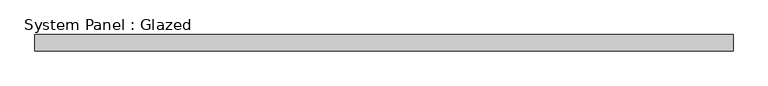
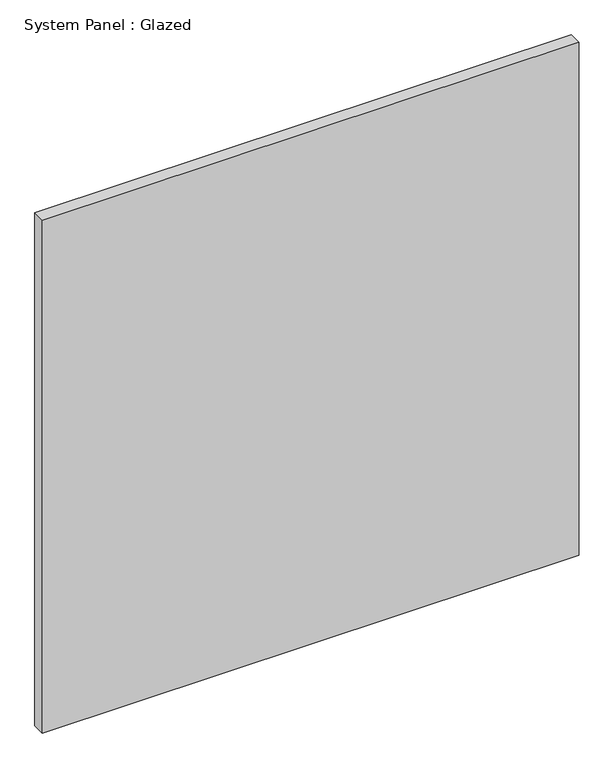
"""IFC4 building model written with IfcOpenShell, lengths in millimetres: plate geometry, System Panel : Glazed."""

from ifc_helpers import new_model, si_unit, origin, origin_with_axes, place, context, project, spatial, polyline, outline, extrude, source, transform, mapped, element, save


def system_panel_glazed_bea6ef26(model_context):
    return source(origin(), model_context, "Body", "SweptSolid", [
        extrude(outline(polyline([(528.0, 24.5), (-528.0, 24.5), (-528.0, 49.5), (528.0, 49.5), (528.0, 24.5)])), origin_with_axes(), (0.0, 0.0, 1.0), 1066.8),
    ])


if __name__ == "__main__":
    model = new_model("IFC4")
    model_context = context("Model", 3, world=origin())
    ifc_project = project(units=[si_unit("LENGTHUNIT", "METRE", prefix="MILLI")], contexts=[model_context])
    site = spatial("IfcSite", under=ifc_project)
    building = spatial("IfcBuilding", under=site)
    placement = place(None, origin())
    system_panel_glazed_shape = system_panel_glazed_bea6ef26(model_context)
    element("IfcPlate", 1, ObjectType="System Panel : Glazed", at=placement, inside=building, context=model_context, shape_type="MappedRepresentation", body=[
        mapped(system_panel_glazed_shape, transform((0.0, 0.0, 0.0), x_axis=(1.0, 0.0, 0.0), y_axis=(0.0, 1.0, 0.0), z_axis=(0.0, 0.0, 1.0))),
    ])
    save(model, "model.ifc")

# Revit data of these elements
# Type "System Panel : Glazed"
#   Construction Type Id = "GSP4R"
#   Analytic Construction = "1/8 in Pilkington single glazing"
#   Visual Light Transmittance = 0.9
#   Solar Heat Gain Coefficient = 0.86
#   Heat Transfer Coefficient (U) = 6.7069 W/(m²·K)
#   Define Thermal Properties by = 1
# Element 1 (IfcPlate, "System Panel : Glazed")
#   Materials on its faces: "Glass"
# Materials
#   "Glass": class "Glass", colour RGB 0 128 192, transparency 0.9, Description = "Soda Lime Glass", Cost = 0
